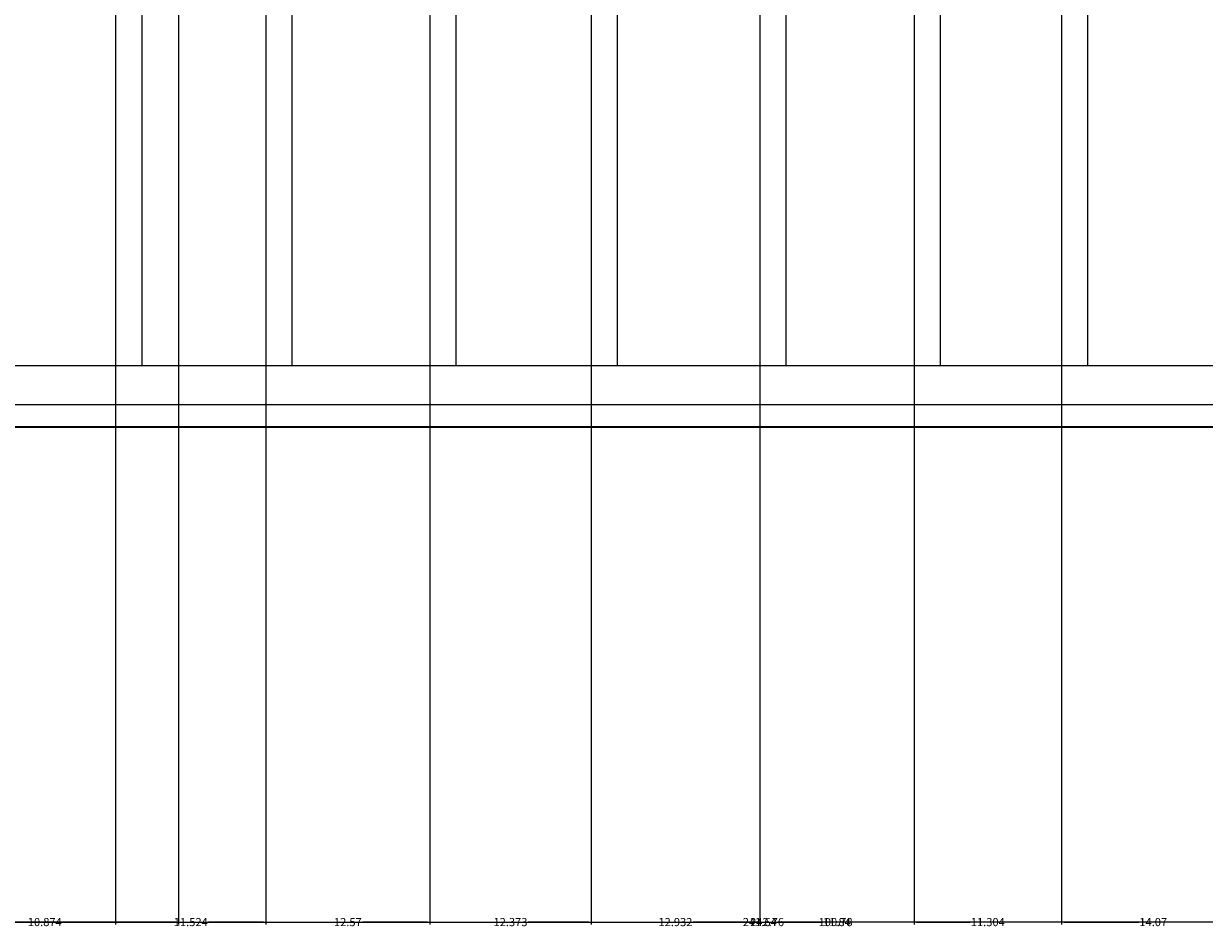
# Model space of a CAD drawing. Units: inches. Extents: x -13 to 809, y 112 to 656.
# Tile 20 of 55: x 430 to 521, y 112 to 181. Entities that reach past the tile are written whole.
import ezdxf

# ---------------------------------------------------------------- set-up
doc = ezdxf.new("R2010")
doc.units = ezdxf.units.IN
doc.header["$MEASUREMENT"] = 0
for name, color, linetype, lineweight in [('A-ANNO-DIMS', 2, 'Continuous', 18), ('A-DOOR', 4, 'Continuous', 25), ('A-ELEV', 7, 'Continuous', 35)]:
    doc.layers.add(name, color=color, linetype=linetype, lineweight=lineweight)
doc.styles.get("Standard").update_dxf_attribs({"font": 'arial.ttf'})
doc.dimstyles.get("Standard").update_dxf_attribs({"dimtxt": 0.625, "dimasz": 0.18, "dimexe": 0.18, "dimexo": 0.0625, "dimgap": 0.09, "dimtad": 0, "dimtih": 1, "dimtoh": 1, "dimdec": 4, "dimzin": 0, "dimdsep": 46, "dimlunit": 4, "dimtxsty": 'Standard', "dimcen": 0.09, "dimadec": 0, "dimazin": 0, "dimtfac": 1, "dimtdec": 4, "dimtofl": 0, "dimtmove": 0, "dimatfit": 3, "dimfxl": 1, "dimtolj": 1, "dimtzin": 0, "dimarcsym": 0})

# ---------------------------------------------------------------- blocks, each defined once
blk = doc.blocks.new('*D20')
at = {"layer": 'A-ANNO-DIMS', "color": 0, "lineweight": -2, "transparency": 16777216}
for p, q in [((365.938, 210.722), (365.938, 112.34)), ((607.574, 209.813), (607.574, 112.34)), ((366.118, 112.52), (485.365, 112.52)), ((607.394, 112.52), (488.148, 112.52))]:
    blk.add_line(p, q, dxfattribs=at)
at = {"layer": 'A-ANNO-DIMS', "color": 0, "transparency": 16777216}
for points in [[(366.118, 112.55), (366.118, 112.49), (365.938, 112.52)], [(607.394, 112.55), (607.394, 112.49), (607.574, 112.52)]]:
    blk.add_solid(points, dxfattribs=at)
at = {"layer": 'Defpoints', "color": 0, "transparency": 16777216}
for p in [(365.938, 210.785), (607.574, 209.875), (607.574, 112.52)]:
    blk.add_point(p, dxfattribs=at)
at = {"layer": 'A-ANNO-DIMS', "color": 0, "transparency": 16777216, "insert": (486.756, 112.52), "char_height": 0.625, "attachment_point": 5}
blk.add_mtext('\\A1;241.64', dxfattribs=at)
blk = doc.blocks.new('*D51')
at = {"layer": 'A-ANNO-DIMS', "color": 0, "lineweight": -2, "transparency": 16777216}
for p, q in [((341.407, 288.388), (341.407, 112.34)), ((442.184, 288.388), (442.184, 112.34)), ((341.587, 112.52), (390.437, 112.52)), ((442.004, 112.52), (393.154, 112.52))]:
    blk.add_line(p, q, dxfattribs=at)
at = {"layer": 'A-ANNO-DIMS', "color": 0, "transparency": 16777216}
for points in [[(341.587, 112.55), (341.587, 112.49), (341.407, 112.52)], [(442.004, 112.55), (442.004, 112.49), (442.184, 112.52)]]:
    blk.add_solid(points, dxfattribs=at)
at = {"layer": 'Defpoints', "color": 0, "transparency": 16777216}
for p in [(341.407, 288.451), (442.184, 288.451), (442.184, 112.52)]:
    blk.add_point(p, dxfattribs=at)
at = {"layer": 'A-ANNO-DIMS', "color": 0, "transparency": 16777216, "insert": (391.796, 112.52), "char_height": 0.625, "attachment_point": 5}
blk.add_mtext('\\A1;100.78', dxfattribs=at)
blk = doc.blocks.new('*D52')
at = {"layer": 'A-ANNO-DIMS', "color": 0, "lineweight": -2, "transparency": 16777216}
for p, q in [((442.184, 288.388), (442.184, 112.34)), ((542.962, 288.388), (542.962, 112.34)), ((442.364, 112.52), (491.215, 112.52)), ((542.782, 112.52), (493.932, 112.52))]:
    blk.add_line(p, q, dxfattribs=at)
at = {"layer": 'A-ANNO-DIMS', "color": 0, "transparency": 16777216}
for points in [[(442.364, 112.55), (442.364, 112.49), (442.184, 112.52)], [(542.782, 112.55), (542.782, 112.49), (542.962, 112.52)]]:
    blk.add_solid(points, dxfattribs=at)
at = {"layer": 'Defpoints', "color": 0, "transparency": 16777216}
for p in [(442.184, 288.451), (542.962, 288.451), (542.962, 112.52)]:
    blk.add_point(p, dxfattribs=at)
at = {"layer": 'A-ANNO-DIMS', "color": 0, "transparency": 16777216, "insert": (492.573, 112.52), "char_height": 0.625, "attachment_point": 5}
blk.add_mtext('\\A1;100.78', dxfattribs=at)
blk = doc.blocks.new('*D130')
at = {"layer": 'A-ANNO-DIMS', "color": 0, "lineweight": -2, "transparency": 16777216}
for p, q in [((365.938, 152.152), (365.938, 112.34)), ((608.694, 150.457), (608.694, 112.34)), ((366.118, 112.52), (485.924, 112.52)), ((608.514, 112.52), (488.709, 112.52))]:
    blk.add_line(p, q, dxfattribs=at)
at = {"layer": 'A-ANNO-DIMS', "color": 0, "transparency": 16777216}
for points in [[(366.118, 112.55), (366.118, 112.49), (365.938, 112.52)], [(608.514, 112.55), (608.514, 112.49), (608.694, 112.52)]]:
    blk.add_solid(points, dxfattribs=at)
at = {"layer": 'Defpoints', "color": 0, "transparency": 16777216}
for p in [(365.938, 152.214), (608.694, 150.52), (608.694, 112.52)]:
    blk.add_point(p, dxfattribs=at)
at = {"layer": 'A-ANNO-DIMS', "color": 0, "transparency": 16777216, "insert": (487.316, 112.52), "char_height": 0.625, "attachment_point": 5}
blk.add_mtext('\\A1;242.76', dxfattribs=at)
blk = doc.blocks.new('*D141')
at = {"layer": 'A-ANNO-DIMS', "color": 0, "lineweight": -2, "transparency": 16777216}
for p, q in [((426.484, 155.152), (426.484, 112.34)), ((437.358, 155.152), (437.358, 112.34)), ((426.664, 112.52), (430.564, 112.52)), ((437.178, 112.52), (433.278, 112.52))]:
    blk.add_line(p, q, dxfattribs=at)
at = {"layer": 'A-ANNO-DIMS', "color": 0, "transparency": 16777216}
for points in [[(426.664, 112.55), (426.664, 112.49), (426.484, 112.52)], [(437.178, 112.55), (437.178, 112.49), (437.358, 112.52)]]:
    blk.add_solid(points, dxfattribs=at)
at = {"layer": 'Defpoints', "color": 0, "transparency": 16777216}
for p in [(426.484, 155.214), (437.358, 155.214), (437.358, 112.52)]:
    blk.add_point(p, dxfattribs=at)
at = {"layer": 'A-ANNO-DIMS', "color": 0, "transparency": 16777216, "insert": (431.921, 112.52), "char_height": 0.625, "attachment_point": 5}
blk.add_mtext('\\A1;10.874', dxfattribs=at)
blk = doc.blocks.new('*D142')
at = {"layer": 'A-ANNO-DIMS', "color": 0, "lineweight": -2, "transparency": 16777216}
for p, q in [((437.358, 155.152), (437.358, 112.34)), ((448.882, 155.152), (448.882, 112.34)), ((437.538, 112.52), (441.763, 112.52)), ((448.702, 112.52), (444.476, 112.52))]:
    blk.add_line(p, q, dxfattribs=at)
at = {"layer": 'A-ANNO-DIMS', "color": 0, "transparency": 16777216}
for points in [[(437.538, 112.55), (437.538, 112.49), (437.358, 112.52)], [(448.702, 112.55), (448.702, 112.49), (448.882, 112.52)]]:
    blk.add_solid(points, dxfattribs=at)
at = {"layer": 'Defpoints', "color": 0, "transparency": 16777216}
for p in [(437.358, 155.214), (448.882, 155.214), (448.882, 112.52)]:
    blk.add_point(p, dxfattribs=at)
at = {"layer": 'A-ANNO-DIMS', "color": 0, "transparency": 16777216, "insert": (443.12, 112.52), "char_height": 0.625, "attachment_point": 5}
blk.add_mtext('\\A1;11.524', dxfattribs=at)
blk = doc.blocks.new('*D143')
at = {"layer": 'A-ANNO-DIMS', "color": 0, "lineweight": -2, "transparency": 16777216}
for p, q in [((448.882, 155.152), (448.882, 112.34)), ((461.451, 155.152), (461.451, 112.34)), ((449.062, 112.52), (454.051, 112.52)), ((461.271, 112.52), (456.281, 112.52))]:
    blk.add_line(p, q, dxfattribs=at)
at = {"layer": 'A-ANNO-DIMS', "color": 0, "transparency": 16777216}
for points in [[(449.062, 112.55), (449.062, 112.49), (448.882, 112.52)], [(461.271, 112.55), (461.271, 112.49), (461.451, 112.52)]]:
    blk.add_solid(points, dxfattribs=at)
at = {"layer": 'Defpoints', "color": 0, "transparency": 16777216}
for p in [(448.882, 155.214), (461.451, 155.214), (461.451, 112.52)]:
    blk.add_point(p, dxfattribs=at)
at = {"layer": 'A-ANNO-DIMS', "color": 0, "transparency": 16777216, "insert": (455.166, 112.52), "char_height": 0.625, "attachment_point": 5}
blk.add_mtext('\\A1;12.57', dxfattribs=at)
blk = doc.blocks.new('*D144')
at = {"layer": 'A-ANNO-DIMS', "color": 0, "lineweight": -2, "transparency": 16777216}
for p, q in [((461.451, 155.152), (461.451, 112.34)), ((473.824, 155.152), (473.824, 112.34)), ((461.631, 112.52), (466.28, 112.52)), ((473.644, 112.52), (468.995, 112.52))]:
    blk.add_line(p, q, dxfattribs=at)
at = {"layer": 'A-ANNO-DIMS', "color": 0, "transparency": 16777216}
for points in [[(461.631, 112.55), (461.631, 112.49), (461.451, 112.52)], [(473.644, 112.55), (473.644, 112.49), (473.824, 112.52)]]:
    blk.add_solid(points, dxfattribs=at)
at = {"layer": 'Defpoints', "color": 0, "transparency": 16777216}
for p in [(461.451, 155.214), (473.824, 155.214), (473.824, 112.52)]:
    blk.add_point(p, dxfattribs=at)
at = {"layer": 'A-ANNO-DIMS', "color": 0, "transparency": 16777216, "insert": (467.638, 112.52), "char_height": 0.625, "attachment_point": 5}
blk.add_mtext('\\A1;12.373', dxfattribs=at)
blk = doc.blocks.new('*D145')
at = {"layer": 'A-ANNO-DIMS', "color": 0, "lineweight": -2, "transparency": 16777216}
for p, q in [((473.824, 155.152), (473.824, 112.34)), ((486.756, 155.152), (486.756, 112.34)), ((474.004, 112.52), (478.935, 112.52)), ((486.576, 112.52), (481.645, 112.52))]:
    blk.add_line(p, q, dxfattribs=at)
at = {"layer": 'A-ANNO-DIMS', "color": 0, "transparency": 16777216}
for points in [[(474.004, 112.55), (474.004, 112.49), (473.824, 112.52)], [(486.576, 112.55), (486.576, 112.49), (486.756, 112.52)]]:
    blk.add_solid(points, dxfattribs=at)
at = {"layer": 'Defpoints', "color": 0, "transparency": 16777216}
for p in [(473.824, 155.214), (486.756, 155.214), (486.756, 112.52)]:
    blk.add_point(p, dxfattribs=at)
at = {"layer": 'A-ANNO-DIMS', "color": 0, "transparency": 16777216, "insert": (480.29, 112.52), "char_height": 0.625, "attachment_point": 5}
blk.add_mtext('\\A1;12.932', dxfattribs=at)
blk = doc.blocks.new('*D146')
at = {"layer": 'A-ANNO-DIMS', "color": 0, "lineweight": -2, "transparency": 16777216}
for p, q in [((486.756, 155.152), (486.756, 112.34)), ((498.596, 155.152), (498.596, 112.34)), ((486.936, 112.52), (491.562, 112.52)), ((498.416, 112.52), (493.79, 112.52))]:
    blk.add_line(p, q, dxfattribs=at)
at = {"layer": 'A-ANNO-DIMS', "color": 0, "transparency": 16777216}
for points in [[(486.936, 112.55), (486.936, 112.49), (486.756, 112.52)], [(498.416, 112.55), (498.416, 112.49), (498.596, 112.52)]]:
    blk.add_solid(points, dxfattribs=at)
at = {"layer": 'Defpoints', "color": 0, "transparency": 16777216}
for p in [(486.756, 155.214), (498.596, 155.214), (498.596, 112.52)]:
    blk.add_point(p, dxfattribs=at)
at = {"layer": 'A-ANNO-DIMS', "color": 0, "transparency": 16777216, "insert": (492.676, 112.52), "char_height": 0.625, "attachment_point": 5}
blk.add_mtext('\\A1;11.84', dxfattribs=at)
blk = doc.blocks.new('*D147')
at = {"layer": 'A-ANNO-DIMS', "color": 0, "lineweight": -2, "transparency": 16777216}
for p, q in [((498.596, 155.152), (498.596, 112.34)), ((509.9, 155.152), (509.9, 112.34)), ((498.776, 112.52), (502.891, 112.52)), ((509.72, 112.52), (505.604, 112.52))]:
    blk.add_line(p, q, dxfattribs=at)
at = {"layer": 'A-ANNO-DIMS', "color": 0, "transparency": 16777216}
for points in [[(498.776, 112.55), (498.776, 112.49), (498.596, 112.52)], [(509.72, 112.55), (509.72, 112.49), (509.9, 112.52)]]:
    blk.add_solid(points, dxfattribs=at)
at = {"layer": 'Defpoints', "color": 0, "transparency": 16777216}
for p in [(498.596, 155.214), (509.9, 155.214), (509.9, 112.52)]:
    blk.add_point(p, dxfattribs=at)
at = {"layer": 'A-ANNO-DIMS', "color": 0, "transparency": 16777216, "insert": (504.248, 112.52), "char_height": 0.625, "attachment_point": 5}
blk.add_mtext('\\A1;11.304', dxfattribs=at)
blk = doc.blocks.new('*D148')
at = {"layer": 'A-ANNO-DIMS', "color": 0, "lineweight": -2, "transparency": 16777216}
for p, q in [((509.9, 155.152), (509.9, 112.34)), ((523.971, 155.152), (523.971, 112.34)), ((510.08, 112.52), (515.82, 112.52)), ((523.791, 112.52), (518.05, 112.52))]:
    blk.add_line(p, q, dxfattribs=at)
at = {"layer": 'A-ANNO-DIMS', "color": 0, "transparency": 16777216}
for points in [[(510.08, 112.55), (510.08, 112.49), (509.9, 112.52)], [(523.791, 112.55), (523.791, 112.49), (523.971, 112.52)]]:
    blk.add_solid(points, dxfattribs=at)
at = {"layer": 'Defpoints', "color": 0, "transparency": 16777216}
for p in [(509.9, 155.214), (523.971, 155.214), (523.971, 112.52)]:
    blk.add_point(p, dxfattribs=at)
at = {"layer": 'A-ANNO-DIMS', "color": 0, "transparency": 16777216, "insert": (516.935, 112.52), "char_height": 0.625, "attachment_point": 5}
blk.add_mtext('\\A1;14.07', dxfattribs=at)

msp = doc.modelspace()

# ---------------------------------------------------------------- linework, layer by layer
at = {"layer": 'A-DOOR'}
for p, q in [((448.8817, 207.4727), (448.8817, 155.2141)), ((450.8817, 207.4652), (450.8817, 155.2141)), ((473.8241, 207.3788), (473.8241, 155.2141)), ((437.3579, 207.3724), (437.3579, 155.2141)), ((439.3579, 207.3724), (439.3579, 155.2141)), ((461.451, 207.3724), (461.451, 155.2141)), ((463.451, 207.3724), (463.451, 155.2141)), ((475.8241, 207.3713), (475.8241, 155.2141)), ((486.7562, 207.3724), (486.7562, 155.2141)), ((488.7562, 207.3724), (488.7562, 155.2141)), ((498.5957, 207.2855), (498.5957, 155.2141)), ((500.5957, 207.278), (500.5957, 155.2141)), ((509.8998, 207.243), (509.8998, 155.2141)), ((511.8998, 207.2355), (511.8998, 155.2141))]:
    msp.add_line(p, q, dxfattribs=at)
for points in [[(365.9383, 210.7849), (607.5741, 209.8753), (607.5741, 152.2141), (365.9383, 152.2141)], [(368.9383, 207.7736), (604.5741, 206.8866), (604.5741, 155.2141), (368.9383, 155.2141)]]:
    msp.add_lwpolyline(points, close=True, dxfattribs=at)
at = {"layer": 'A-ELEV'}
msp.add_line((109.5888, 150.5199), (649.5888, 150.5199), dxfattribs=at)

# ---------------------------------------------------------------- dimensions: what is measured, and where the dimension line sits
at = {"layer": 'A-ANNO-DIMS'}
for base, p1, p2, override, picture, middle in [((442.1845, 112.5199), (341.4072, 288.4508), (442.1845, 288.4508), {"dimdec": 2, "dimlfac": 1, "dimrnd": 0, "dimzin": 0, "dimdsep": 46, "dimlunit": 2}, '*D51', (391.7958, 112.5199)), ((542.9617, 112.5199), (442.1845, 288.4508), (542.9617, 288.4508), {"dimdec": 2, "dimlfac": 1, "dimrnd": 0, "dimzin": 0, "dimdsep": 46, "dimlunit": 2}, '*D52', (492.5731, 112.5199)), ((607.5741, 112.5199), (365.9383, 210.7849), (607.5741, 209.8753), {"dimdec": 2, "dimlfac": 1, "dimrnd": 0, "dimzin": 0, "dimdsep": 46, "dimlunit": 2}, '*D20', (486.7562, 112.5199)), ((437.3579, 112.5199), (426.484, 155.2141), (437.3579, 155.2141), {"dimdec": 3, "dimlfac": 1, "dimrnd": 0, "dimzin": 0, "dimdsep": 46, "dimlunit": 2}, '*D141', (431.9209, 112.5199)), ((448.8817, 112.5199), (437.3579, 155.2141), (448.8817, 155.2141), {"dimdec": 3, "dimlfac": 1, "dimrnd": 0, "dimzin": 0, "dimdsep": 46, "dimlunit": 2}, '*D142', (443.1198, 112.5199)), ((461.451, 112.5199), (448.8817, 155.2141), (461.451, 155.2141), {"dimdec": 2, "dimlfac": 1, "dimrnd": 0, "dimzin": 0, "dimdsep": 46, "dimlunit": 2}, '*D143', (455.1663, 112.5199)), ((473.8241, 112.5199), (461.451, 155.2141), (473.8241, 155.2141), {"dimdec": 3, "dimlfac": 1, "dimrnd": 0, "dimzin": 0, "dimdsep": 46, "dimlunit": 2}, '*D144', (467.6375, 112.5199)), ((486.7562, 112.5199), (473.8241, 155.2141), (486.7562, 155.2141), {"dimdec": 3, "dimlfac": 1, "dimrnd": 0, "dimzin": 0, "dimdsep": 46, "dimlunit": 2}, '*D145', (480.2901, 112.5199)), ((498.5957, 112.5199), (486.7562, 155.2141), (498.5957, 155.2141), {"dimdec": 2, "dimlfac": 1, "dimrnd": 0, "dimzin": 0, "dimdsep": 46, "dimlunit": 2}, '*D146', (492.6759, 112.5199)), ((509.8998, 112.5199), (498.5957, 155.2141), (509.8998, 155.2141), {"dimdec": 3, "dimlfac": 1, "dimrnd": 0, "dimzin": 0, "dimdsep": 46, "dimlunit": 2}, '*D147', (504.2477, 112.5199)), ((523.9709, 112.5199), (509.8998, 155.2141), (523.9709, 155.2141), {"dimdec": 2, "dimlfac": 1, "dimrnd": 0, "dimzin": 0, "dimdsep": 46, "dimlunit": 2}, '*D148', (516.9353, 112.5199)), ((608.694, 112.5199), (365.9383, 152.2141), (608.694, 150.5199), {"dimdec": 2, "dimlfac": 1, "dimrnd": 0, "dimzin": 0, "dimdsep": 46, "dimlunit": 2}, '*D130', (487.3161, 112.5199))]:
    dim = msp.add_linear_dim(base=base, p1=p1, p2=p2, dimstyle='Standard', override=override, dxfattribs=at)
    dim.commit()
    dim.dimension.update_dxf_attribs({"geometry": picture, "text_midpoint": middle})

doc.saveas('drawing.dxf')
